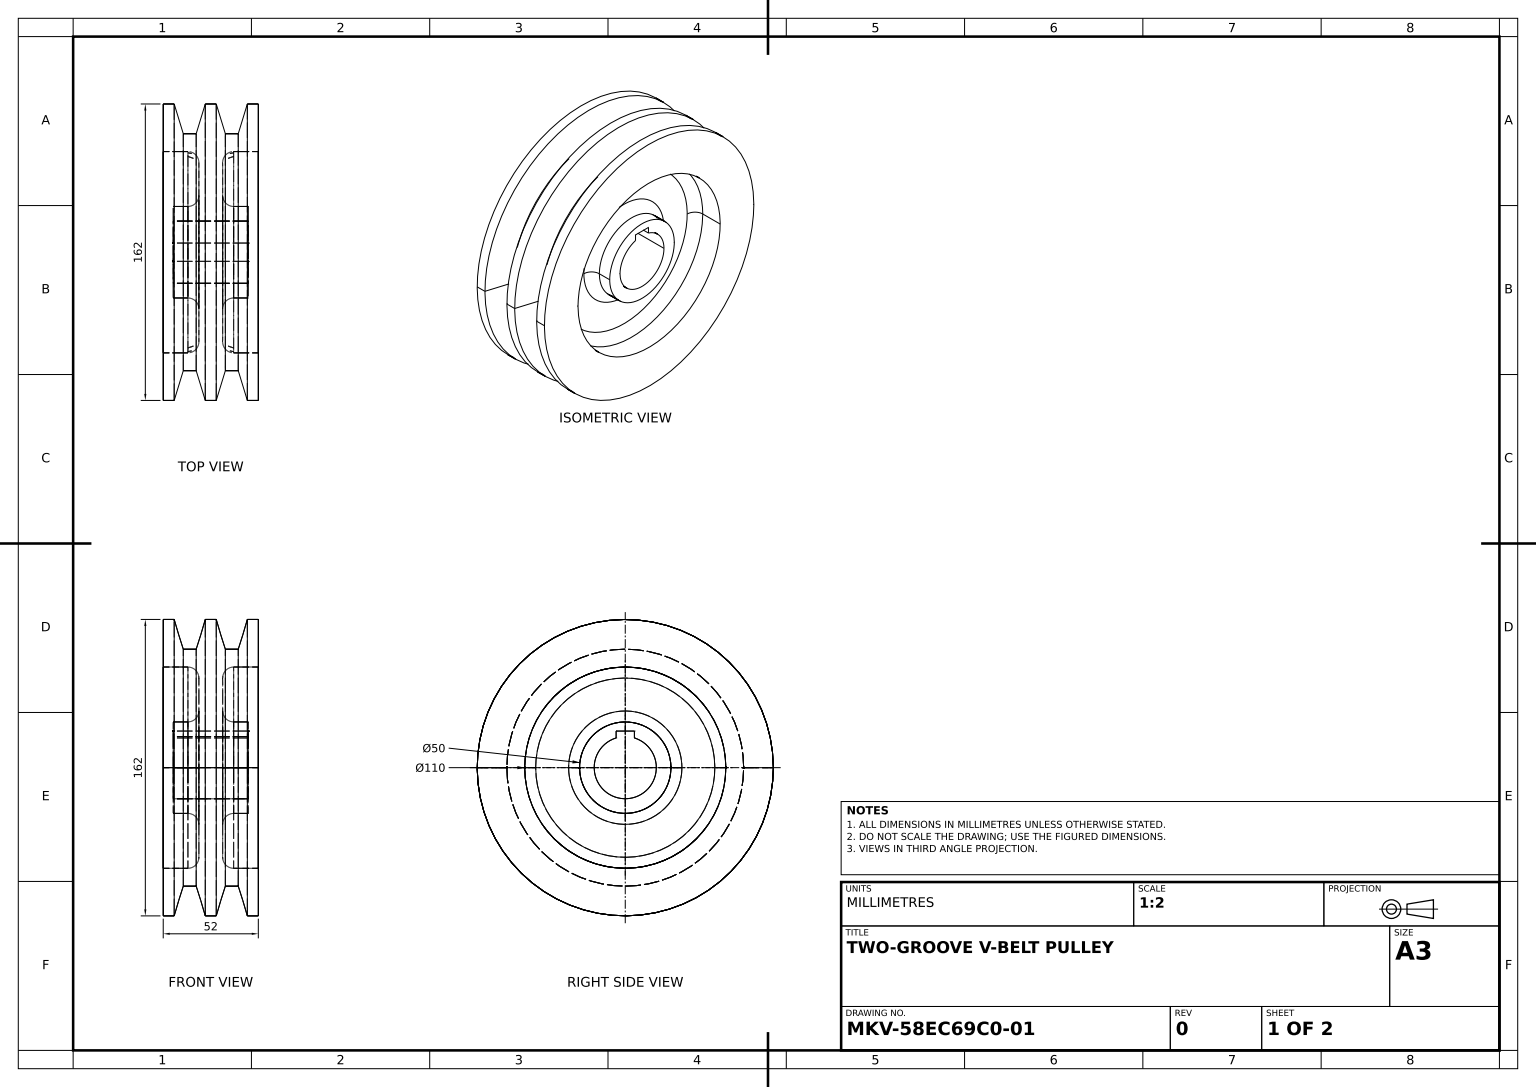
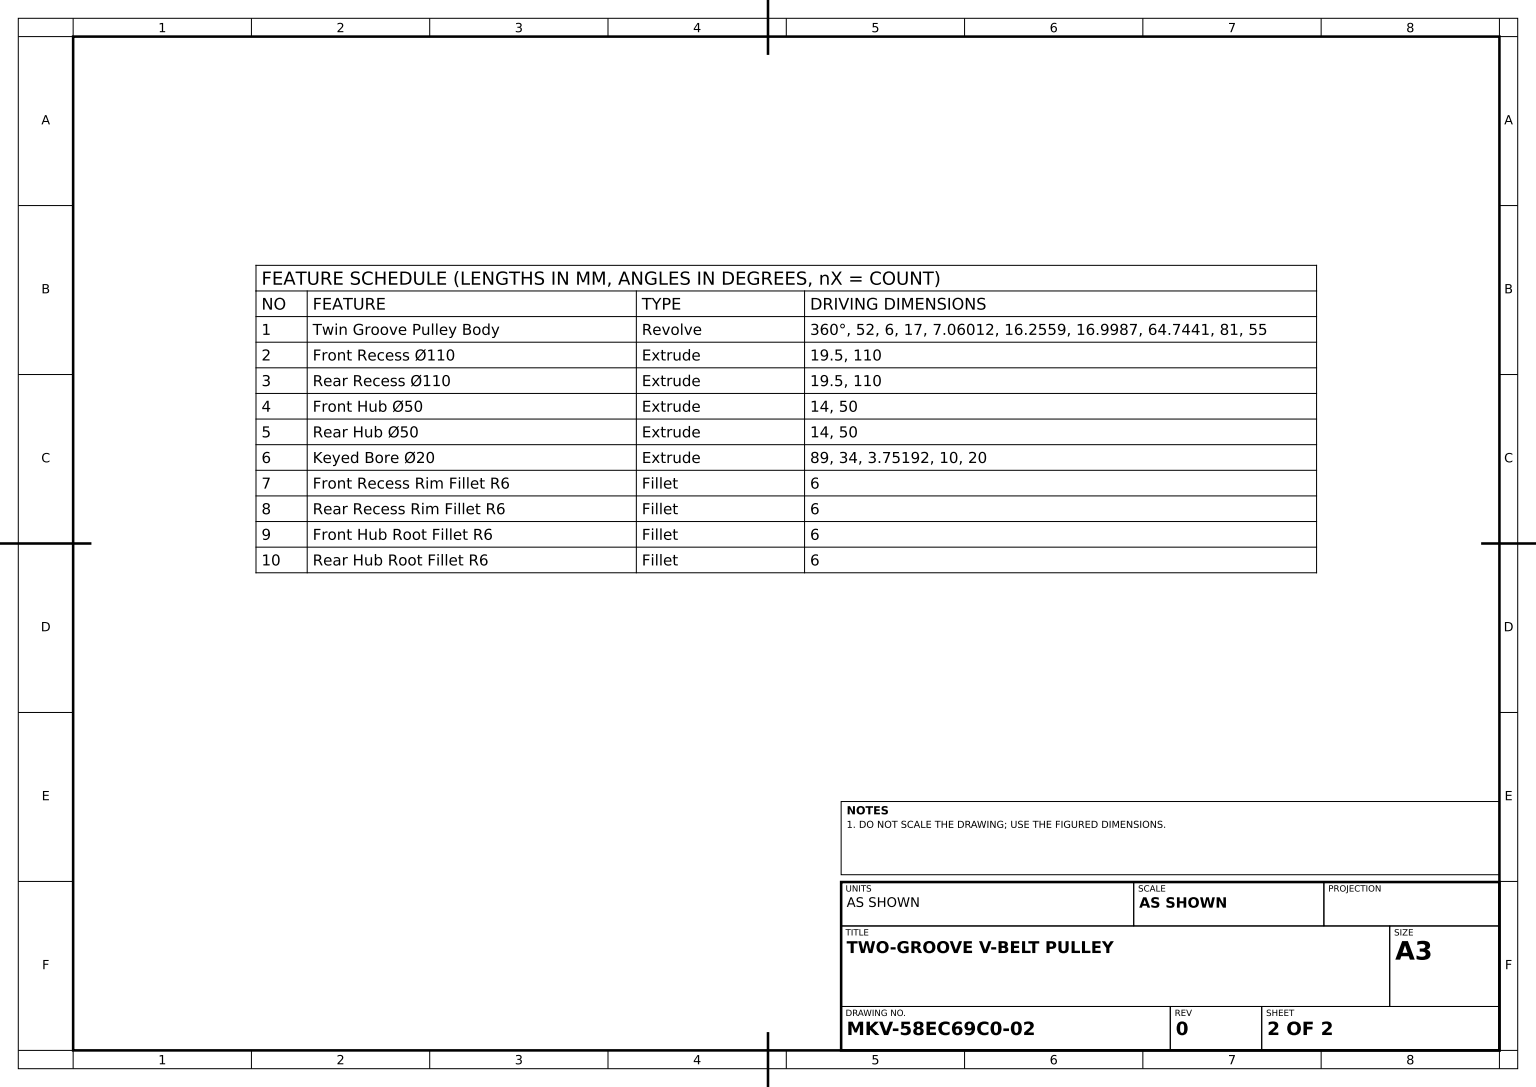
SolidWorks part; units mm, degrees
material "Plain Carbon Steel"
ref_plane "Front Plane" through (0, 0, 0) normal (0, 0, 1) x (1, 0, 0)
ref_plane "Top Plane" through (0, 0, 0) normal (0, 1, 0) x (1, 0, 0)
ref_plane "Right Plane" through (0, 0, 0) normal (1, 0, 0) x (0, 0, -1)
sketch "Pulley Rim Profile Sketch" plane through (0, 0, 0) normal (0, 0, 1) x (1, 0, 0)
  line L0 (0, 0) -> (0, 81)
  line L1 (0, 81) -> (6, 81)
  line L3 (23, 81) -> (18.0301, 64.7441)
  line L4 (6, 81) -> (10.9699, 64.7441)
  line L5 (0, 0) -> (0, 55)
  line L7 (10.9699, 64.7441) -> (18.0301, 64.7441)
  line L8 (23, 81) -> (29, 81)
  line L9 (29, 81) -> (33.9699, 64.7441)
  line L10 (46, 81) -> (52, 81)
  line L11 (46, 81) -> (41.0301, 64.7441)
  line L12 (33.9699, 64.7441) -> (41.0301, 64.7441)
  line L13 (52, 81) -> (52, 0)
  line L14 (52, 0) -> (0, 0)
  dimension "D1" = 52
  dimension "D2" = 6
  dimension "D3" = 17
  dimension "D4" = 6
  dimension "D5" = 6
  dimension "D6" = 7.0601
  dimension "D7" = 16.2559
  dimension "D8" = 64.7441
  dimension "D9" = 64.7441
  dimension "D10" = 81
  dimension "D11" = 81
  dimension "D12" = 16.9987
  dimension "D13" = 16.9987
  dimension "D14" = 55
revolve "Twin Groove Pulley Body" add sketch "Pulley Rim Profile Sketch" angle 360 about L14
sketch "Front Recess Ø110 Sketch" plane through (52, 0, 0) normal (1, 0, 0) x (0, 0, -1)
  circle A0 centre (0, 0) radius 55
  dimension "D1" = 110
extrude "Front Recess Ø110" cut sketch "Front Recess Ø110 Sketch" against normal blind 19.5
sketch "Rear Recess Ø110 Sketch" plane through (0, 0, 0) normal (-1, 0, 0) x (0, 0, 1)
  circle A0 centre (0, 0) radius 55
  dimension "D1" = 110
extrude "Rear Recess Ø110" cut sketch "Rear Recess Ø110 Sketch" against normal blind 19.5
sketch "Front Hub Ø50 Sketch" plane through (32.5, 0, 0) normal (1, 0, 0) x (0, 0, -1)
  circle A0 centre (0, 0) radius 25
  dimension "D1" = 50
extrude "Front Hub Ø50" add sketch "Front Hub Ø50 Sketch" along normal blind 14
sketch "Rear Hub Ø50 Sketch" plane through (19.5, 0, 0) normal (-1, 0, 0) x (0, 0, 1)
  circle A0 centre (0, 0) radius 25
  dimension "D1" = 50
extrude "Rear Hub Ø50" add sketch "Rear Hub Ø50 Sketch" along normal blind 14
sketch "Keyed Bore Ø20 Sketch" plane through (5.5, 0, 0) normal (-1, 0, 0) x (0, 0, 1)
  line L1 (0, 20) -> (5, 20)
  line L2 (5, 20) -> (5, 16.2481)
  line L4 (-5, 16.2481) -> (-5, 20)
  line L5 (-5, 20) -> (0, 20)
  arc A0 (-5, 16.2481) -> (5, 16.2481) centre (0, 0) ccw
  dimension "D1" = 34
  dimension "D2" = 3.7519
  dimension "D3" = 10
  dimension "D4" = 3.7519
  dimension "D5" = 20
extrude "Keyed Bore Ø20" cut sketch "Keyed Bore Ø20 Sketch" against normal blind 89
fillet "Front Recess Rim Fillet R6" radius 6 1 edges at (32.5, 0, -55)
fillet "Rear Recess Rim Fillet R6" radius 6 1 edges at (19.5, 0, 55)
fillet "Front Hub Root Fillet R6" radius 6 1 edges at (32.5, 0, -25)
fillet "Rear Hub Root Fillet R6" radius 6 1 edges at (19.5, 0, 25)
